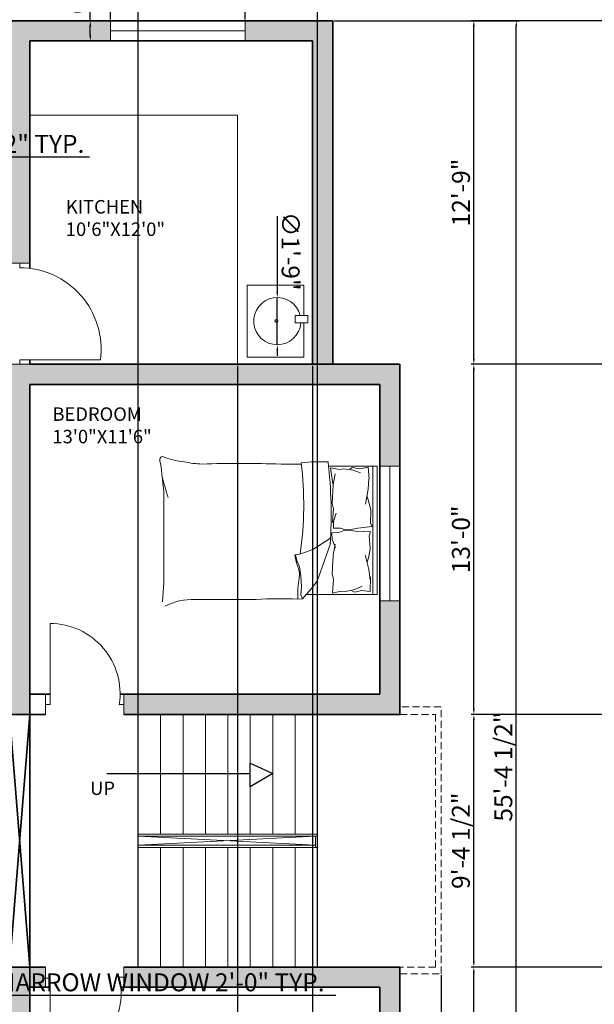
# Model space of a CAD drawing. Units: inches. Extents: x 2257 to 3678, y 834 to 1975.
# Tile 5 of 16: x 2696 to 2952, y 1155 to 1594. Entities that reach past the tile are written whole.
import ezdxf

# ---------------------------------------------------------------- set-up
doc = ezdxf.new("R2010")
doc.units = ezdxf.units.IN
doc.linetypes.add('HIDDEN2', pattern=[4.7625, 3.175, -1.5875])
for name, color, linetype, lineweight in [('A-ANNO-DIMS', 2, 'Continuous', 18), ('A-ANNO-SYMB', 7, 'Continuous', 25), ('A-ANNO-TEXT', 7, 'Continuous', 18), ('A-AREA-IDEN', 7, 'Continuous', 18), ('A-DOOR', 3, 'Continuous', 18), ('A-FLOR-CASE', 8, 'Continuous', 18), ('A-FLOR-FIXT', 9, 'Continuous', 18), ('A-FLOR-OVHD', 254, 'HIDDEN2', 13), ('A-FLOR-STRS', 7, 'Continuous', 18), ('A-FURN', 8, 'Continuous', 18), ('A-GLAZ', 4, 'Continuous', 18), ('A-WALL', 7, 'Continuous', 35)]:
    doc.layers.add(name, color=color, linetype=linetype, lineweight=lineweight)
doc.layers.add('A-WALL-PATT', color=251, linetype='Continuous', lineweight=13, true_color=0x636466)
doc.styles.get("Standard").update_dxf_attribs({"font": 'arial.ttf'})
doc.dimstyles.new('ISO-25', dxfattribs={"dimtxt": 8, "dimasz": 2.5, "dimexe": 1.25, "dimexo": 0.625, "dimtad": 1, "dimdec": 0, "dimlunit": 3, "dimtxsty": 'Standard', "dimcen": 2.5, "dimadec": 0, "dimazin": 0, "dimtfac": 1, "dimtdec": 0, "dimtmove": 0, "dimatfit": 3, "dimfxl": 1, "dimarcsym": 0})

# ---------------------------------------------------------------- blocks, each defined once
blk = doc.blocks.new('BED-DOUBLE-PLAN')
for p, q in [((0, 61.46), (31.9, 61.46)), ((0, 4.17), (0, 61.46)), ((1.84, 4.17), (1.84, 61.46)), ((33.26, 63.38), (29.37, 58.94)), ((35.36, 63.48), (33.26, 63.38, 4.64)), ((34.01, 61.54), (33.26, 63.38)), ((33.63, 57.82), (34.01, 61.54)), ((3.07, 60.08), (2.95, 53.6)), ((3.07, 60.08), (6.92, 59.62)), ((9.9, 59.11), (6.69, 57.7)), ((6.92, 59.62), (10, 60.34)), ((14.18, 60.08), (9.9, 59.11)), ((10, 60.34), (11.25, 59.72)), ((16.11, 59.85), (14.18, 60.08)), ((19.87, 60.78), (16.11, 59.85)), ((19.38, 54.63), (19.87, 60.78)), ((29.37, 58.94), (26.77, 55.41)), ((34.01, 53.18), (33.63, 57.82)), ((2.95, 53.6), (3.05, 54.8)), ((3.05, 54.8), (3.68, 50.25)), ((20.05, 52.28), (19.38, 54.63)), ((26.77, 55.41), (24.36, 48.73)), ((34.56, 49.1), (34.01, 53.18)), ((3.68, 50.25), (5.3, 43.75)), ((19.54, 43.87), (20.05, 52.28)), ((24.36, 48.73), (20.84, 38.73)), ((35.68, 46.68), (34.56, 49.1)), ((3.69, 44.52), (3.04, 41.01)), ((4.4, 47), (3.69, 44.52)), ((18.74, 39.04), (19.54, 43.87)), ((36.42, 43.71), (35.68, 46.68)), ((95, 18.06), (95, 47.57)), ((3.04, 41.01), (3.07, 40.62)), ((3.07, 40.62), (3.57, 35.31)), ((20.07, 36.86), (18.53, 40.55)), ((20.84, 36.28), (28.62, 41.3)), ((28.62, 41.3), (34.01, 43.34)), ((34.01, 43.34), (36.42, 43.71)), ((3.57, 35.31), (2.99, 33.54)), ((20.25, 33.92), (20.07, 36.86)), ((2.24, 31.15), (8.66, 31.84)), ((2.94, 29.42), (2.24, 31.15)), ((2.99, 33.54), (9.43, 33.25)), ((8.66, 31.84), (12.47, 32.54)), ((9.43, 33.25), (13.28, 32.79)), ((12.47, 32.54), (14.03, 32.54)), ((13.28, 32.79), (14.84, 32.89)), ((14.03, 32.54), (16.28, 31.84)), ((14.84, 32.89), (17.04, 33.72)), ((16.28, 31.84), (19.5, 31.84)), ((17.04, 33.72), (20.25, 33.92)), ((19.5, 31.84), (19.5, 28.9)), ((2.76, 24.09), (2.94, 29.42)), ((19.5, 28.9), (18.19, 25.13)), ((19.38, 23.24), (19.87, 29.39)), ((2.76, 23.7), (2.76, 24.09)), ((3.63, 20.23), (2.76, 23.7)), ((20.05, 20.89), (19.38, 23.24)), ((4.5, 17.81), (3.63, 20.23)), ((3.98, 14.52), (5.19, 21.1)), ((19.54, 12.48), (20.05, 20.89)), ((3.63, 9.93), (3.98, 14.52)), ((3.61, 9.81), (3.63, 9.93)), ((4, 4.67), (3.61, 9.81)), ((18.74, 7.65), (19.54, 12.48)), ((19.54, 12.48), (19.92, 11.13)), ((19.92, 11.13), (20.79, 5.02)), ((3.98, 4.67), (7.79, 5.36)), ((10.74, 6.06), (7.44, 7.27)), ((7.79, 5.36), (10.91, 4.84)), ((15.07, 5.36), (10.74, 6.06)), ((10.91, 4.84), (12.12, 5.54)), ((16.98, 5.71), (15.07, 5.36)), ((20.79, 5.02), (16.98, 5.71)), ((21.71, 4.17), (0, 4.17))]:
    blk.add_line(p, q)
for centre, radius, start, end in [((82.32, 91.3), 27.65, 267.4714, 296.4681), ((-7.98, 61.53), 43.38, 349.8763, 2.5657), ((43.54, 218.51), 155.25, 266.9791, 273.8365), ((81.31, -5405.34), 5469.02, 90.00217, 90.28689), ((254.49, 49.33), 159.5, 174.4998, 180.6351), ((42.04, 52.44), 7.46, 168.6608, 203.7384), ((1.78, 37.35), 35.55, 10.6617, 19.8806), ((36.49, 43.92), 0.221, 250.2464, 1.1377), ((187.4, 21.29), 154.68, 171.7845, 186.9006), ((218.26, 25.61), 197.77, 176.0865, 186.7821), ((-28.43, -20.65), 127.63, 13.3832, 17.7053), ((240.78, 25.69), 145.97, 182.9958, 189.4091), ((24.09, 102.1), 99.87, 268.7218, 275.604), ((37.37, -200.58), 203.94, 88.4762, 91.0082), ((60.68, 581.23), 578.22, 268.22771, 271.71854), ((77.34, -32.25), 35.53, 76.0648, 88.9113), ((84.25, -25.97), 28.25, 67.9751, 86.652), ((95.57, 1.3), 1.31, 236.1736, 23.4781)]:
    blk.add_arc(centre, radius, start, end)
blk = doc.blocks.new('WIN-60')
for p, q in [((0, 9), (0, 0)), ((60, 4.5), (60, 9)), ((60, 9), (60, 0)), ((0, 0), (0, 4.5)), ((0, 4.5), (60, 4.5))]:
    blk.add_line(p, q)
blk = doc.blocks.new('DOOR-KITCHEN')
for p, q in [((0, 45), (9, 45)), ((4.5, 45), (4.5, 43)), ((9, 45), (4.5, 45)), ((4.5, 0), (4.5, 2)), ((4.5, 2), (40.5, 2)), ((9, 0), (0, 0))]:
    blk.add_line(p, q)
blk.add_arc((4.5, 6.7), 36.3, 352.5694, 90)
blk = doc.blocks.new('DOOR-BEDROOM-EAST')
for p, q in [((2, 4.5), (2, 40.5)), ((0, 9), (0, 0)), ((34.84, 0), (34.84, 9)), ((34.84, 9), (34.84, 4.5)), ((0, 4.5), (2, 4.5)), ((34.84, 4.5), (32.84, 4.5))]:
    blk.add_line(p, q)
blk.add_arc((2, 9.29), 31.21, 351.1699, 90)
blk = doc.blocks.new('DOOR-BEDROOM-FRONT')
for p, q in [((0, 41.01), (0, 32.01)), ((34.84, 41.01), (34.84, 32.01)), ((0, 36.08), (2, 36.08)), ((2, 36.08), (2, 0.08)), ((34.84, 36.51), (32.84, 36.51)), ((34.84, 32.01), (34.84, 36.51))]:
    blk.add_line(p, q)
blk.add_arc((4.15, 29.52), 29.53, 265.822, 13.6871)
blk = doc.blocks.new('*D50')
at = {"layer": 'A-ANNO-DIMS', "color": 0, "lineweight": -2, "transparency": 16777216}
for p, q in [((2603.02, 1531.36), (2603.02, 1534.2)), ((2605.52, 1532.95), (2615.26, 1532.95)), ((2617.76, 1531.36), (2617.76, 1534.2)), ((2617.76, 1532.95), (2726.7, 1532.95))]:
    blk.add_line(p, q, dxfattribs=at)
at = {"layer": 'A-ANNO-DIMS', "color": 0, "transparency": 16777216}
for points in [[(2605.52, 1533.37), (2605.52, 1532.53), (2603.02, 1532.95)], [(2615.26, 1533.37), (2615.26, 1532.53), (2617.76, 1532.95)]]:
    blk.add_solid(points, dxfattribs=at)
at = {"layer": 'Defpoints', "color": 0, "transparency": 16777216}
for p in [(2603.02, 1530.74), (2617.76, 1532.95), (2617.76, 1530.74)]:
    blk.add_point(p, dxfattribs=at)
at = {"layer": 'A-ANNO-DIMS', "color": 0, "transparency": 16777216, "insert": (2673.48, 1537.71), "char_height": 8, "attachment_point": 5}
blk.add_mtext('CHAIR 1\'-2 1/2" TYP.', dxfattribs=at)
blk = doc.blocks.new('*D56')
at = {"layer": 'A-ANNO-DIMS', "color": 0, "lineweight": -2, "transparency": 16777216}
for p, q in [((2736.02, 1594.2), (2736.02, 1603.83)), ((2738.52, 1602.58), (2793.52, 1602.58)), ((2796.02, 1594.2), (2796.02, 1603.83)), ((2796.02, 1602.58), (2901, 1602.58))]:
    blk.add_line(p, q, dxfattribs=at)
at = {"layer": 'A-ANNO-DIMS', "color": 0, "transparency": 16777216}
for points in [[(2738.52, 1602.99), (2738.52, 1602.16), (2736.02, 1602.58)], [(2793.52, 1602.99), (2793.52, 1602.16), (2796.02, 1602.58)]]:
    blk.add_solid(points, dxfattribs=at)
at = {"layer": 'Defpoints', "color": 0, "transparency": 16777216}
for p in [(2796.02, 1602.58), (2736.02, 1593.58), (2796.02, 1593.58)]:
    blk.add_point(p, dxfattribs=at)
at = {"layer": 'A-ANNO-DIMS', "color": 0, "transparency": 16777216, "insert": (2849.76, 1607.34), "char_height": 8, "attachment_point": 5}
blk.add_mtext('WINDOW 5\'-0" TYP.', dxfattribs=at)
blk = doc.blocks.new('*D57')
at = {"layer": 'A-ANNO-DIMS', "color": 0, "lineweight": -2, "transparency": 16777216}
for p, q in [((2727.02, 1593.58), (2727.02, 1646.09)), ((2735.39, 1593.58), (2725.77, 1593.58)), ((2727.02, 1587.08), (2727.02, 1591.08)), ((2735.39, 1584.58), (2725.77, 1584.58))]:
    blk.add_line(p, q, dxfattribs=at)
at = {"layer": 'A-ANNO-DIMS', "color": 0, "transparency": 16777216}
for points in [[(2726.6, 1591.08), (2727.44, 1591.08), (2727.02, 1593.58)], [(2726.6, 1587.08), (2727.44, 1587.08), (2727.02, 1584.58)]]:
    blk.add_solid(points, dxfattribs=at)
at = {"layer": 'Defpoints', "color": 0, "transparency": 16777216}
for p in [(2727.02, 1593.58), (2736.02, 1593.58), (2736.02, 1584.58)]:
    blk.add_point(p, dxfattribs=at)
at = {"layer": 'A-ANNO-DIMS', "color": 0, "transparency": 16777216, "insert": (2722.31, 1621.08), "char_height": 8, "attachment_point": 5, "rotation": 90}
blk.add_mtext('0\'-9" TYP.', dxfattribs=at)
blk = doc.blocks.new('*D60')
at = {"layer": 'A-ANNO-DIMS', "color": 0, "lineweight": -2, "transparency": 16777216}
for p, q in [((2654.22, 1162.45), (2654.22, 1158.23)), ((2678.22, 1162.45), (2678.22, 1158.23)), ((2656.72, 1159.48), (2675.72, 1159.48)), ((2678.22, 1159.48), (2836.5, 1159.48))]:
    blk.add_line(p, q, dxfattribs=at)
at = {"layer": 'A-ANNO-DIMS', "color": 0, "transparency": 16777216}
for points in [[(2656.72, 1159.89), (2656.72, 1159.06), (2654.22, 1159.48)], [(2675.72, 1159.89), (2675.72, 1159.06), (2678.22, 1159.48)]]:
    blk.add_solid(points, dxfattribs=at)
at = {"layer": 'Defpoints', "color": 0, "transparency": 16777216}
for p in [(2654.22, 1163.08), (2678.22, 1163.08), (2678.22, 1159.48)]:
    blk.add_point(p, dxfattribs=at)
at = {"layer": 'A-ANNO-DIMS', "color": 0, "transparency": 16777216, "insert": (2758.61, 1164.24), "char_height": 8, "attachment_point": 5}
blk.add_mtext('NARROW WINDOW 2\'-0" TYP.', dxfattribs=at)
blk = doc.blocks.new('*D96')
at = {"layer": 'A-ANNO-DIMS', "color": 0, "lineweight": -2, "transparency": 16777216}
for p, q in [((2337.05, 1283.95), (2337.05, 894.3)), ((2883.34, 1168.45), (2883.34, 894.3)), ((2339.55, 895.55), (2880.84, 895.55))]:
    blk.add_line(p, q, dxfattribs=at)
at = {"layer": 'A-ANNO-DIMS', "color": 0, "transparency": 16777216}
for points in [[(2339.55, 895.97), (2339.55, 895.14), (2337.05, 895.55)], [(2880.84, 895.97), (2880.84, 895.14), (2883.34, 895.55)]]:
    blk.add_solid(points, dxfattribs=at)
at = {"layer": 'Defpoints', "color": 0, "transparency": 16777216}
for p in [(2337.05, 1284.58), (2883.34, 1169.08), (2883.34, 895.55)]:
    blk.add_point(p, dxfattribs=at)
at = {"layer": 'A-ANNO-DIMS', "color": 0, "transparency": 16777216, "insert": (2610.2, 900.31), "char_height": 8, "attachment_point": 5}
blk.add_mtext('45\'-6 1/2"', dxfattribs=at)
blk = doc.blocks.new('*D97')
at = {"layer": 'A-ANNO-DIMS', "color": 0, "lineweight": -2, "transparency": 16777216}
for p, q in [((2835.68, 1593.58), (2918.14, 1593.58)), ((2916.89, 931.6), (2916.89, 1591.08)), ((2700.87, 929.1), (2918.14, 929.1))]:
    blk.add_line(p, q, dxfattribs=at)
at = {"layer": 'A-ANNO-DIMS', "color": 0, "transparency": 16777216}
for points in [[(2916.47, 1591.08), (2917.31, 1591.08), (2916.89, 1593.58)], [(2916.47, 931.6), (2917.31, 931.6), (2916.89, 929.1)]]:
    blk.add_solid(points, dxfattribs=at)
at = {"layer": 'Defpoints', "color": 0, "transparency": 16777216}
for p in [(2835.05, 1593.58), (2916.89, 1593.58), (2700.25, 929.1)]:
    blk.add_point(p, dxfattribs=at)
at = {"layer": 'A-ANNO-DIMS', "color": 0, "transparency": 16777216, "insert": (2912.13, 1261.34), "char_height": 8, "attachment_point": 5, "rotation": 90}
blk.add_mtext('55\'-4 1/2"', dxfattribs=at)
blk = doc.blocks.new('*D101')
at = {"layer": 'A-ANNO-DIMS', "color": 0, "lineweight": -2, "transparency": 16777216}
for p, q in [((3136.62, 1172.08), (2896.72, 1172.08)), ((2897.97, 1012.58), (2897.97, 1169.58)), ((3010.62, 1010.08), (2896.72, 1010.08))]:
    blk.add_line(p, q, dxfattribs=at)
at = {"layer": 'A-ANNO-DIMS', "color": 0, "transparency": 16777216}
for points in [[(2897.55, 1169.58), (2898.38, 1169.58), (2897.97, 1172.08)], [(2897.55, 1012.58), (2898.38, 1012.58), (2897.97, 1010.08)]]:
    blk.add_solid(points, dxfattribs=at)
at = {"layer": 'Defpoints', "color": 0, "transparency": 16777216}
for p in [(2897.97, 1172.08), (3137.24, 1172.08), (3011.24, 1010.08)]:
    blk.add_point(p, dxfattribs=at)
at = {"layer": 'A-ANNO-DIMS', "color": 0, "transparency": 16777216, "insert": (2893.25, 1091.08), "char_height": 8, "attachment_point": 5, "rotation": 90}
blk.add_mtext('13\'-6"', dxfattribs=at)
blk = doc.blocks.new('*D102')
at = {"layer": 'A-ANNO-DIMS', "color": 0, "lineweight": -2, "transparency": 16777216}
for p, q in [((2980.62, 1284.58), (2896.72, 1284.58)), ((2897.97, 1174.58), (2897.97, 1282.08)), ((3136.62, 1172.08), (2896.72, 1172.08))]:
    blk.add_line(p, q, dxfattribs=at)
at = {"layer": 'A-ANNO-DIMS', "color": 0, "transparency": 16777216}
for points in [[(2897.55, 1282.08), (2898.38, 1282.08), (2897.97, 1284.58)], [(2897.55, 1174.58), (2898.38, 1174.58), (2897.97, 1172.08)]]:
    blk.add_solid(points, dxfattribs=at)
at = {"layer": 'Defpoints', "color": 0, "transparency": 16777216}
for p in [(2897.97, 1284.58), (2981.24, 1284.58), (3137.24, 1172.08)]:
    blk.add_point(p, dxfattribs=at)
at = {"layer": 'A-ANNO-DIMS', "color": 0, "transparency": 16777216, "insert": (2893.21, 1228.33), "char_height": 8, "attachment_point": 5, "rotation": 90}
blk.add_mtext('9\'-4 1/2"', dxfattribs=at)
blk = doc.blocks.new('*D103')
at = {"layer": 'A-ANNO-DIMS', "color": 0, "lineweight": -2, "transparency": 16777216}
for p, q in [((2980.62, 1440.58), (2896.72, 1440.58)), ((2897.97, 1287.08), (2897.97, 1438.08)), ((2980.62, 1284.58), (2896.72, 1284.58))]:
    blk.add_line(p, q, dxfattribs=at)
at = {"layer": 'A-ANNO-DIMS', "color": 0, "transparency": 16777216}
for points in [[(2897.55, 1438.08), (2898.38, 1438.08), (2897.97, 1440.58)], [(2897.55, 1287.08), (2898.38, 1287.08), (2897.97, 1284.58)]]:
    blk.add_solid(points, dxfattribs=at)
at = {"layer": 'Defpoints', "color": 0, "transparency": 16777216}
for p in [(2897.97, 1440.58), (2981.24, 1440.58), (2981.24, 1284.58)]:
    blk.add_point(p, dxfattribs=at)
at = {"layer": 'A-ANNO-DIMS', "color": 0, "transparency": 16777216, "insert": (2893.25, 1362.58), "char_height": 8, "attachment_point": 5, "rotation": 90}
blk.add_mtext('13\'-0"', dxfattribs=at)
blk = doc.blocks.new('*D104')
at = {"layer": 'A-ANNO-DIMS', "color": 0, "lineweight": -2, "transparency": 16777216}
for p, q in [((3010.62, 1593.58), (2896.72, 1593.58)), ((2897.97, 1443.08), (2897.97, 1591.08)), ((2980.62, 1440.58), (2896.72, 1440.58))]:
    blk.add_line(p, q, dxfattribs=at)
at = {"layer": 'A-ANNO-DIMS', "color": 0, "transparency": 16777216}
for points in [[(2897.55, 1591.08), (2898.38, 1591.08), (2897.97, 1593.58)], [(2897.55, 1443.08), (2898.38, 1443.08), (2897.97, 1440.58)]]:
    blk.add_solid(points, dxfattribs=at)
at = {"layer": 'Defpoints', "color": 0, "transparency": 16777216}
for p in [(2897.97, 1593.58), (3011.24, 1593.58), (2981.24, 1440.58)]:
    blk.add_point(p, dxfattribs=at)
at = {"layer": 'A-ANNO-DIMS', "color": 0, "transparency": 16777216, "insert": (2893.26, 1517.08), "char_height": 8, "attachment_point": 5, "rotation": 90}
blk.add_mtext('12\'-9"', dxfattribs=at)
blk = doc.blocks.new('*D113')
at = {"layer": 'A-ANNO-DIMS', "color": 0, "lineweight": -2, "transparency": 16777216}
for p, q in [((2748.35, 1172.7), (2748.35, 1628.38)), ((2828.35, 1172.7), (2828.35, 1628.38)), ((2750.85, 1627.13), (2825.85, 1627.13))]:
    blk.add_line(p, q, dxfattribs=at)
at = {"layer": 'A-ANNO-DIMS', "color": 0, "transparency": 16777216}
for points in [[(2750.85, 1627.54), (2750.85, 1626.71), (2748.35, 1627.13)], [(2825.85, 1627.54), (2825.85, 1626.71), (2828.35, 1627.13)]]:
    blk.add_solid(points, dxfattribs=at)
at = {"layer": 'Defpoints', "color": 0, "transparency": 16777216}
for p in [(2828.35, 1627.13), (2748.35, 1172.08), (2828.35, 1172.08)]:
    blk.add_point(p, dxfattribs=at)
at = {"layer": 'A-ANNO-DIMS', "color": 0, "transparency": 16777216, "insert": (2788.35, 1631.84), "char_height": 8, "attachment_point": 5}
blk.add_mtext('6\'-8"', dxfattribs=at)
blk = doc.blocks.new('*D117')
at = {"layer": 'A-ANNO-DIMS', "color": 0, "lineweight": -2, "transparency": 16777216}
for p, q in [((2792.7, 1439.95), (2792.7, 894.3)), ((2826.05, 1439.95), (2826.05, 894.3)), ((2792.7, 895.55), (2748.91, 895.55)), ((2823.55, 895.55), (2795.2, 895.55))]:
    blk.add_line(p, q, dxfattribs=at)
at = {"layer": 'A-ANNO-DIMS', "color": 0, "transparency": 16777216}
for points in [[(2795.2, 895.97), (2795.2, 895.14), (2792.7, 895.55)], [(2823.55, 895.97), (2823.55, 895.14), (2826.05, 895.55)]]:
    blk.add_solid(points, dxfattribs=at)
at = {"layer": 'Defpoints', "color": 0, "transparency": 16777216}
for p in [(2792.7, 1440.58), (2826.05, 1440.58), (2792.7, 895.55)]:
    blk.add_point(p, dxfattribs=at)
at = {"layer": 'A-ANNO-DIMS', "color": 0, "transparency": 16777216, "insert": (2769.55, 900.31), "char_height": 8, "attachment_point": 5}
blk.add_mtext('2\'-9 1/2"', dxfattribs=at)
blk = doc.blocks.new('*D150')
at = {"layer": 'A-ANNO-DIMS', "color": 0, "lineweight": -2, "transparency": 16777216}
for p, q in [((2810.31, 1506.52), (2810.35, 1472.8)), ((2810.37, 1449.28), (2810.35, 1470.3)), ((2810.38, 1446.78), (2810.38, 1444.28))]:
    blk.add_line(p, q, dxfattribs=at)
at = {"layer": 'A-ANNO-DIMS', "color": 0, "transparency": 16777216}
for points in [[(2810.76, 1472.8), (2809.93, 1472.8), (2810.35, 1470.3)], [(2810.79, 1446.78), (2809.96, 1446.78), (2810.37, 1449.28)]]:
    blk.add_solid(points, dxfattribs=at)
at = {"layer": 'Defpoints', "color": 0, "transparency": 16777216}
for p in [(2810.35, 1470.3), (2810.37, 1449.28)]:
    blk.add_point(p, dxfattribs=at)
at = {"layer": 'A-ANNO-DIMS', "color": 0, "transparency": 16777216, "insert": (2815.26, 1490.92), "char_height": 8, "attachment_point": 5, "rotation": 270.0675}
blk.add_mtext('∅1\'-9"', dxfattribs=at)

msp = doc.modelspace()

# ---------------------------------------------------------------- hatches: boundary and pattern name
at = {"layer": 'A-WALL-PATT'}
h = msp.add_hatch(color=256, dxfattribs=at)
h.dxf.hatch_style = 1
h.paths.add_polyline_path([(2736.02, 1589.08), (2736.02, 1593.58), (2691.05, 1593.58), (2648.2, 1593.58), (2648.2, 1584.58), (2691.05, 1584.58), (2691.05, 1485.58), (2700.05, 1485.58), (2700.05, 1584.58), (2736.02, 1584.58)])
h.paths.add_polyline_path([(2835.05, 1593.58), (2796.02, 1593.58), (2796.02, 1584.58), (2826.05, 1584.58), (2826.05, 1440.58), (2835.05, 1440.58)])
h.paths.add_polyline_path([(2865.05, 1440.58), (2826.05, 1440.58), (2700.05, 1440.58), (2691.05, 1440.58), (2691.05, 1431.58), (2691.05, 1284.58), (2700.05, 1284.58), (2700.05, 1431.58), (2826.05, 1431.58), (2856.05, 1431.58), (2856.05, 1395.2), (2865.05, 1395.2), (2865.05, 1431.58)])
h.paths.add_polyline_path([(2865.05, 1335.2), (2856.05, 1335.2), (2856.05, 1293.58), (2741.94, 1293.58), (2741.94, 1289.08), (2741.94, 1284.58), (2865.05, 1284.58)], flags=17)
h.paths.add_polyline_path([(2865.05, 1172.08), (2856.05, 1172.08), (2741.94, 1172.08), (2741.94, 1163.08), (2856.05, 1163.08), (2856.05, 1133.53), (2865.05, 1133.53)])
h.paths.add_polyline_path([(2865.05, 1073.53), (2856.05, 1073.53), (2856.05, 1019.08), (2795.28, 1019.08), (2795.28, 1010.08), (2865.05, 1010.08)])
h.paths.add_polyline_path([(2735.28, 1014.58), (2735.28, 1019.08), (2700.05, 1019.08), (2700.05, 1026.35), (2695.55, 1026.35), (2691.05, 1026.35), (2691.05, 1010.08), (2735.28, 1010.08)])
h.paths.add_polyline_path([(2700.05, 1163.08), (2700.05, 1172.08), (2691.05, 1172.08), (2685.7, 1172.08), (2685.7, 1163.08), (2691.05, 1163.08), (2691.05, 1058.19), (2700.05, 1058.19)])
h.paths.add_polyline_path([(2707.1, 1172.08), (2700.05, 1172.08), (2700.05, 1163.08), (2707.1, 1163.08)])
h.paths.add_polyline_path([(2685.7, 1172.08), (2678.22, 1172.08), (2678.22, 1163.08), (2685.7, 1163.08)])
h.paths.add_polyline_path([(2654.22, 1172.08), (2648.96, 1172.08), (2648.96, 1163.08), (2654.22, 1163.08), (2654.22, 1167.58)])
h.paths.add_polyline_path([(2553.05, 1163.08), (2558.66, 1163.08), (2558.66, 1172.08), (2544.05, 1172.08), (2544.05, 1163.08), (2544.05, 1058.19), (2553.05, 1058.19)])
h.paths.add_polyline_path([(2568.8, 1167.58), (2568.8, 1172.08), (2558.66, 1172.08), (2558.66, 1163.08), (2568.8, 1163.08)])
h.paths.add_polyline_path([(2596.82, 1172.08), (2592.8, 1172.08), (2592.8, 1163.08), (2596.82, 1163.08)])
h.paths.add_polyline_path([(2553.05, 1019.08), (2553.05, 1026.35), (2548.55, 1026.35), (2544.05, 1026.35), (2544.05, 1019.08), (2476.8, 1019.08), (2476.8, 1010.08), (2553.05, 1010.08)])
h.paths.add_polyline_path([(2376.05, 1163.08), (2502.05, 1163.08), (2502.05, 1172.08), (2446.55, 1172.08), (2446.55, 1195.52), (2446.55, 1215.32), (2442.05, 1215.32), (2442.05, 1195.52), (2442.05, 1172.08), (2412.05, 1172.08), (2412.05, 1167.58), (2376.05, 1167.58), (2376.05, 1172.08), (2376.05, 1201.28), (2367.05, 1201.28), (2367.05, 1172.08), (2367.05, 1123.86), (2376.05, 1123.86)])
h.paths.add_polyline_path([(2577.05, 1440.58), (2376.05, 1440.58), (2376.05, 1485.89), (2367.05, 1485.89), (2367.05, 1440.58), (2337.05, 1440.58), (2337.05, 1403.59), (2346.05, 1403.59), (2346.05, 1431.58), (2493.05, 1431.58), (2493.05, 1293.58), (2484.41, 1293.58), (2484.41, 1284.58), (2502.05, 1284.58), (2502.05, 1431.58), (2577.05, 1431.58)])
h.paths.add_polyline_path([(2346.05, 1343.59), (2337.05, 1343.59), (2337.05, 1284.58), (2448.12, 1284.58), (2448.12, 1289.08), (2448.12, 1293.58), (2346.05, 1293.58)], flags=17)
h.paths.add_polyline_path([(2376.05, 1244.08), (2446.55, 1244.08), (2446.55, 1248.58), (2367.05, 1248.58), (2367.05, 1225.28), (2375.64, 1225.28), (2375.64, 1228.02), (2376.05, 1228.02)])
h.paths.add_polyline_path([(2588.2, 1589.08), (2588.2, 1593.58), (2468.1, 1593.58), (2468.1, 1584.58), (2544.05, 1584.58), (2544.05, 1541.08), (2568.05, 1541.08), (2568.05, 1490.08), (2544.05, 1490.08), (2544.05, 1485.58), (2577.05, 1485.58), (2577.05, 1545.58), (2553.05, 1545.58), (2553.05, 1584.58), (2588.2, 1584.58)])
h.paths.add_polyline_path([(2376.05, 1584.58), (2408.1, 1584.58), (2408.1, 1589.08), (2408.1, 1593.58), (2367.05, 1593.58), (2367.05, 1545.89), (2376.05, 1545.89)])
h.paths.add_polyline_path([(2376.05, 1063.86), (2367.05, 1063.86), (2367.05, 1019.08), (2367.05, 1010.08), (2416.8, 1010.08), (2416.8, 1014.58), (2416.8, 1019.08), (2376.05, 1019.08)])

# ---------------------------------------------------------------- linework, layer by layer
at = {"layer": 'A-ANNO-SYMB'}
for p, q in [((2798.35, 1252.32), (2798.35, 1262.82)), ((2798.35, 1262.82), (2808.35, 1258.25)), ((2734.33, 1258.25), (2798.35, 1258.25)), ((2808.35, 1258.25), (2798.35, 1252.32))]:
    msp.add_line(p, q, dxfattribs=at)
at = {"layer": 'A-FLOR-CASE'}
for p, q in [((2700.05, 1551.47), (2792.7, 1551.47)), ((2792.7, 1551.47), (2792.7, 1440.58))]:
    msp.add_line(p, q, dxfattribs=at)
at = {"layer": 'A-FLOR-FIXT'}
msp.add_lwpolyline([(2822.19, 1459), (2822.19, 1443.67), (2796.92, 1443.67), (2796.92, 1475.78), (2822.19, 1475.78), (2822.19, 1462.24)], dxfattribs=at)
msp.add_lwpolyline([(2818.31, 1462.24), (2824.04, 1462.24), (2824.04, 1459), (2818.31, 1459)], close=True, dxfattribs=at)
msp.add_circle((2809.98, 1459.9), 0.685, dxfattribs=at)
msp.add_arc((2810.36, 1459.79), 10.51, 13.5048, 355.6836, dxfattribs=at)
at = {"layer": 'A-FLOR-OVHD'}
for p, q in [((2883.34, 1288.02), (2865.05, 1288.02)), ((2883.34, 1169.08), (2883.34, 1288.02)), ((2865.05, 1284.58), (2880.88, 1284.58)), ((2880.88, 1284.58), (2880.88, 1172.08)), ((2880.88, 1172.08), (2865.05, 1172.08)), ((2865.05, 1172.08), (2865.05, 1169.08)), ((2865.05, 1169.08), (2883.34, 1169.08))]:
    msp.add_line(p, q, dxfattribs=at)
at = {"layer": 'A-FLOR-STRS'}
for p, q in [((2748.35, 1284.58), (2748.35, 1231.33)), ((2758.35, 1284.58), (2758.35, 1231.33)), ((2768.35, 1284.58), (2768.35, 1231.33)), ((2778.35, 1284.58), (2778.35, 1231.33)), ((2788.35, 1284.58), (2788.35, 1231.33)), ((2798.35, 1284.58), (2798.35, 1231.33)), ((2808.35, 1284.58), (2808.35, 1231.33)), ((2818.35, 1284.58), (2818.35, 1231.33)), ((2828.35, 1284.58), (2828.35, 1231.33)), ((2828.35, 1231.33), (2748.35, 1231.33)), ((2748.35, 1231.33), (2748.35, 1230.33)), ((2748.35, 1230.33), (2828.35, 1230.33)), ((2748.35, 1226.33), (2827.35, 1230.33)), ((2827.35, 1226.33), (2748.35, 1230.33)), ((2828.35, 1230.33), (2827.35, 1230.33)), ((2827.35, 1230.33), (2827.35, 1225.77)), ((2827.35, 1230.33), (2827.35, 1226.33)), ((2828.35, 1231.33), (2828.35, 1228.01)), ((2827.35, 1226.33), (2748.35, 1226.33)), ((2748.35, 1226.33), (2748.35, 1225.33)), ((2748.35, 1225.33), (2748.35, 1226.33)), ((2748.35, 1225.33), (2828.35, 1225.33)), ((2748.35, 1225.33), (2748.35, 1172.08)), ((2758.35, 1225.33), (2758.35, 1172.08)), ((2768.35, 1225.33), (2768.35, 1172.08)), ((2778.35, 1225.33), (2778.35, 1172.08)), ((2788.35, 1225.33), (2788.35, 1172.08)), ((2798.35, 1225.33), (2798.35, 1172.08)), ((2808.35, 1225.33), (2808.35, 1172.08)), ((2818.35, 1225.33), (2818.35, 1172.08)), ((2827.35, 1225.33), (2827.35, 1226.33)), ((2827.35, 1225.77), (2827.35, 1225.33)), ((2828.35, 1228.01), (2828.35, 1225.33)), ((2828.35, 1225.33), (2828.35, 1172.08))]:
    msp.add_line(p, q, dxfattribs=at)
at = {"layer": 'A-WALL'}
for p, q in [((2367.05, 1593.58), (2835.05, 1593.58)), ((2691.05, 1593.58), (2835.05, 1593.58)), ((2835.05, 1593.58), (2835.05, 1440.58)), ((2700.05, 1584.58), (2700.05, 1483.3)), ((2700.05, 1584.58), (2826.05, 1584.58)), ((2826.05, 1584.58), (2826.05, 1440.58)), ((2700.05, 1442.58), (2700.05, 1440.58)), ((2700.05, 1440.58), (2826.05, 1440.58)), ((2826.05, 1440.58), (2865.05, 1440.58)), ((2865.05, 1440.58), (2865.05, 1431.58)), ((2700.05, 1431.58), (2700.05, 1172.08)), ((2700.05, 1431.58), (2826.05, 1431.58)), ((2826.05, 1431.58), (2856.05, 1431.58)), ((2856.05, 1431.58), (2856.05, 1293.58)), ((2865.05, 1431.58), (2865.05, 1284.58)), ((2700.05, 1293.58), (2709.1, 1293.58)), ((2740.31, 1293.58), (2856.05, 1293.58)), ((2700.05, 1284.58), (2691.05, 1284.58)), ((2700.05, 1172.08), (2691.05, 1284.58)), ((2691.05, 1284.58), (2700.05, 1284.58)), ((2700.05, 1284.58), (2691.05, 1172.08)), ((2700.05, 1284.58), (2707.1, 1284.58)), ((2741.94, 1284.58), (2865.05, 1284.58)), ((2691.05, 1172.08), (2700.05, 1172.08)), ((2700.05, 1172.08), (2707.1, 1172.08)), ((2700.05, 1172.08), (2700.05, 1163.08)), ((2700.05, 1172.08), (2700.05, 1172.08)), ((2741.94, 1172.08), (2856.05, 1172.08)), ((2856.05, 1172.08), (2865.05, 1172.08)), ((2865.05, 1172.08), (2865.05, 1010.08)), ((2700.05, 1163.08), (2709.1, 1163.08)), ((2700.05, 1163.08), (2700.05, 1055.91)), ((2740.67, 1163.08), (2856.05, 1163.08)), ((2856.05, 1163.08), (2856.05, 1019.08)), ((2856.05, 1163.08), (2856.05, 1019.08))]:
    msp.add_line(p, q, dxfattribs=at)

# ---------------------------------------------------------------- block references
at = {"layer": 'A-DOOR'}
for name, p in [('DOOR-KITCHEN', (2691.05, 1440.58)), ('DOOR-BEDROOM-EAST', (2707.1, 1284.58)), ('DOOR-BEDROOM-FRONT', (2707.1, 1131.07))]:
    msp.add_blockref(name, p, dxfattribs=at)
at = {"layer": 'A-FURN', "rotation": 180}
msp.add_blockref('BED-DOUBLE-PLAN', (2854.86, 1399.42), dxfattribs=at)
at = {"layer": 'A-GLAZ'}
msp.add_blockref('WIN-60', (2736.02, 1584.58), dxfattribs=at)
at = {"layer": 'A-GLAZ', "extrusion": (0, 0, -1), "zscale": -1, "rotation": 269.9999999999991}
msp.add_blockref('WIN-60', (-2865.05, 1395.2), dxfattribs=at)

# ---------------------------------------------------------------- texts
at = {"layer": 'A-ANNO-TEXT', "insert": (2726.93, 1254.72), "char_height": 6, "attachment_point": 1}
msp.add_mtext_dynamic_manual_height_columns('UP', width=36.0702, gutter_width=12.5, heights=[0], dxfattribs=at)
at = {"layer": 'A-AREA-IDEN', "char_height": 6, "attachment_point": 1}
for s, width, insert in [('KITCHEN\\P10\'6"X12\'0"', 183.6078, (2716.11, 1513.73)), ('BEDROOM\\P13\'0"X11\'6"', 186.0434, (2710.15, 1421.37))]:
    msp.add_mtext_dynamic_manual_height_columns(s, width=width, gutter_width=12.5, heights=[0], dxfattribs=dict(at, insert=insert))

# ---------------------------------------------------------------- dimensions: what is measured, and where the dimension line sits
at = {"layer": 'A-ANNO-DIMS'}
for base, p1, p2, angle, text, picture, middle in [((2727.02, 1593.58), (2736.02, 1584.58), (2736.02, 1593.58), 90, '<> TYP.', '*D57', (2722.31, 1621.08)), ((2617.76, 1532.95), (2603.02, 1530.74), (2617.76, 1530.74), 360, 'CHAIR <> TYP.', '*D50', (2673.48, 1537.71))]:
    dim = msp.add_linear_dim(base=base, p1=p1, p2=p2, angle=angle, text=text, dimstyle='ISO-25', override={"dimdec": 1, "dimlfac": 1, "dimrnd": 0, "dimzin": 1, "dimdsep": 46, "dimlunit": 4, "dimfrac": 2}, dxfattribs=at)
    dim.commit()
    dim.dimension.update_dxf_attribs({"geometry": picture, "text_midpoint": middle})
for base, p1, p2, picture, middle in [((2828.35, 1627.13), (2748.35, 1172.08), (2828.35, 1172.08), '*D113', (2788.35, 1631.84)), ((2792.699, 895.5533), (2826.0509, 1440.5769), (2792.699, 1440.5769), '*D117', (2769.5522, 900.3148)), ((2883.34, 895.55), (2337.05, 1284.58), (2883.34, 1169.08), '*D96', (2610.2, 900.31))]:
    dim = msp.add_linear_dim(base=base, p1=p1, p2=p2, dimstyle='ISO-25', override={"dimdec": 1, "dimlfac": 1, "dimrnd": 0, "dimzin": 1, "dimdsep": 46, "dimlunit": 4, "dimfrac": 2}, dxfattribs=at)
    dim.commit()
    dim.dimension.update_dxf_attribs({"geometry": picture, "text_midpoint": middle})
for base, p1, p2, text, picture, middle in [((2796.02, 1602.58), (2736.02, 1593.58), (2796.02, 1593.58), 'WINDOW <> TYP.', '*D56', (2849.76, 1607.34)), ((2678.22, 1159.48), (2654.22, 1163.08), (2678.22, 1163.08), 'NARROW WINDOW <> TYP.', '*D60', (2758.61, 1164.24))]:
    dim = msp.add_linear_dim(base=base, p1=p1, p2=p2, text=text, dimstyle='ISO-25', override={"dimdec": 1, "dimlfac": 1, "dimrnd": 0, "dimzin": 1, "dimdsep": 46, "dimlunit": 4, "dimfrac": 2}, dxfattribs=at)
    dim.commit()
    dim.dimension.update_dxf_attribs({"geometry": picture, "text_midpoint": middle})
for base, p1, p2, picture, middle in [((2916.89, 1593.58), (2700.25, 929.1), (2835.05, 1593.58), '*D97', (2912.13, 1261.34)), ((2897.97, 1593.58), (2981.24, 1440.58), (3011.24, 1593.58), '*D104', (2893.26, 1517.08)), ((2897.97, 1440.58), (2981.24, 1284.58), (2981.24, 1440.58), '*D103', (2893.25, 1362.58)), ((2897.97, 1284.58), (3137.24, 1172.08), (2981.24, 1284.58), '*D102', (2893.21, 1228.33)), ((2897.97, 1172.08), (3011.24, 1010.08), (3137.24, 1172.08), '*D101', (2893.25, 1091.08))]:
    dim = msp.add_linear_dim(base=base, p1=p1, p2=p2, angle=90, dimstyle='ISO-25', override={"dimdec": 1, "dimlfac": 1, "dimrnd": 0, "dimzin": 1, "dimdsep": 46, "dimlunit": 4, "dimfrac": 2}, dxfattribs=at)
    dim.commit()
    dim.dimension.update_dxf_attribs({"geometry": picture, "text_midpoint": middle})
dim = msp.add_diameter_dim_2p(p1=(2810.37, 1449.28), p2=(2810.35, 1470.3), dimstyle='ISO-25', override={"dimdec": 1, "dimlfac": 1, "dimrnd": 0, "dimzin": 1, "dimdsep": 46, "dimlunit": 4, "dimfrac": 2}, dxfattribs=at)
dim.commit()
dim.dimension.update_dxf_attribs({"geometry": '*D150', "text_midpoint": (2810.33, 1490.91)})

doc.saveas('drawing.dxf')
